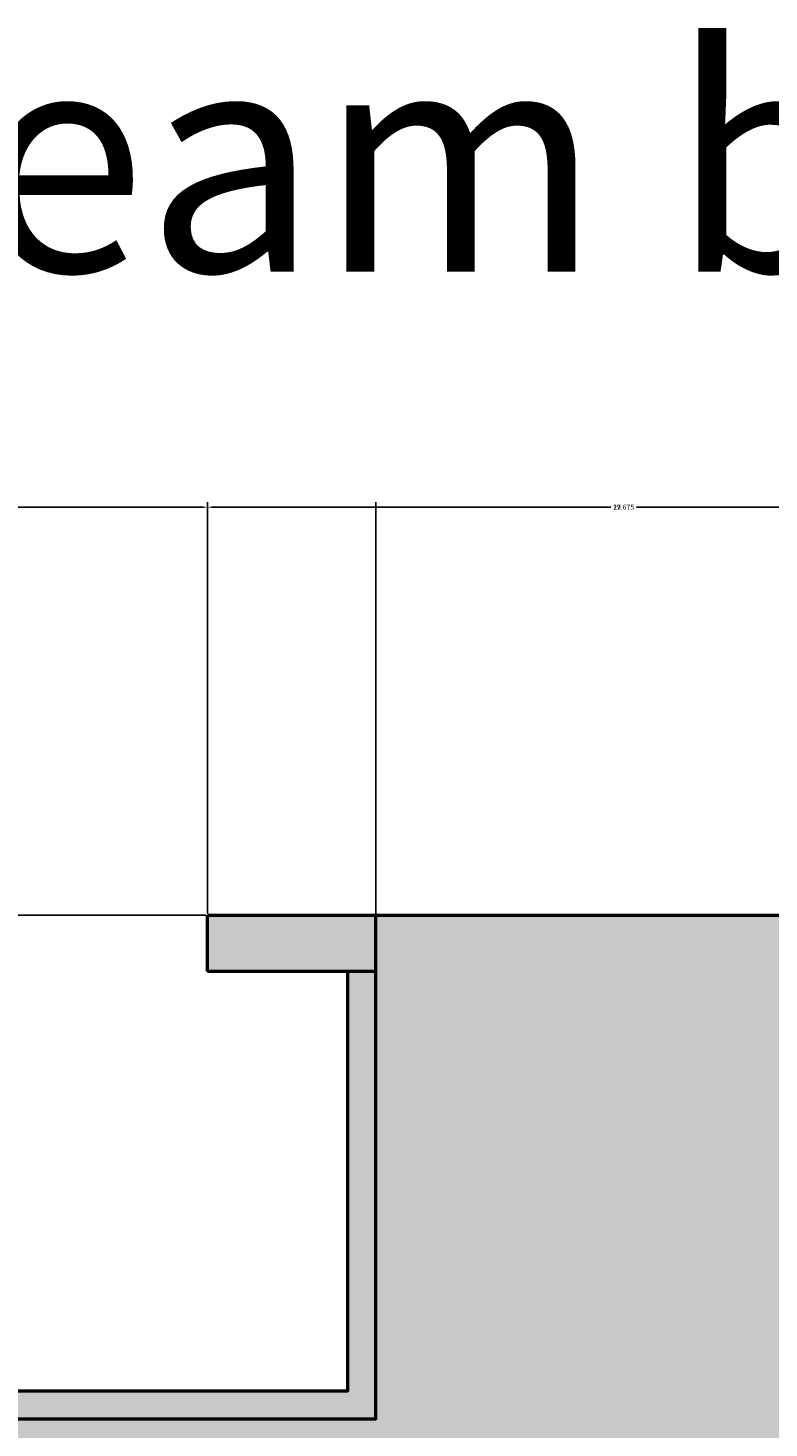
# Model space of a CAD drawing. Units: inches. Extents: x -12 to 334, y -10 to 186.
# Tile 66 of 77: x 184 to 210, y 137 to 186. Entities that reach past the tile are written whole.
import ezdxf

# ---------------------------------------------------------------- set-up
doc = ezdxf.new("R2010")
doc.units = ezdxf.units.IN
doc.header["$MEASUREMENT"] = 0
for name, color, linetype, lineweight in [('M-ANNO-TEXT', 3, 'Continuous', 25), ('M-DIMS', 2, 'Continuous', 18), ('M-EQPM', 7, 'Continuous', 50), ('M-EQPM-PATT', 8, 'Continuous', 18)]:
    doc.layers.add(name, color=color, linetype=linetype, lineweight=lineweight)
doc.styles.get("Standard").update_dxf_attribs({"font": 'arial.ttf'})
doc.dimstyles.get("Standard").update_dxf_attribs({"dimtxt": 0.18, "dimasz": 0.18, "dimexe": 0.18, "dimexo": 0.0625, "dimgap": 0.09, "dimtad": 0, "dimtih": 1, "dimtoh": 1, "dimdec": 4, "dimzin": 0, "dimdsep": 46, "dimtxsty": 'Standard', "dimcen": 0.09, "dimadec": 0, "dimazin": 0, "dimtfac": 1, "dimtdec": 4, "dimtofl": 0, "dimtmove": 0, "dimatfit": 3, "dimfxl": 1, "dimtolj": 1, "dimtzin": 0, "dimarcsym": 0})

# ---------------------------------------------------------------- blocks, each defined once
blk = doc.blocks.new('*D18')
at = {"layer": 'Defpoints', "color": 0, "transparency": 16777216}
for p in [(190.342, 169.385), (190.342, 154.835), (126.379, 137.887)]:
    blk.add_point(p, dxfattribs=at)
at = {"layer": 'M-DIMS', "color": 0, "lineweight": -2, "transparency": 16777216}
for p, q in [((126.379, 137.95), (126.379, 169.565)), ((126.559, 169.385), (157.967, 169.385)), ((190.162, 169.385), (158.755, 169.385)), ((190.342, 154.897), (190.342, 169.565))]:
    blk.add_line(p, q, dxfattribs=at)
at = {"layer": 'M-DIMS', "color": 0, "transparency": 16777216}
for points in [[(126.559, 169.415), (126.559, 169.355), (126.379, 169.385)], [(190.162, 169.415), (190.162, 169.355), (190.342, 169.385)]]:
    blk.add_solid(points, dxfattribs=at)
at = {"layer": 'M-DIMS', "color": 0, "transparency": 16777216, "insert": (158.361, 169.385), "char_height": 0.18, "attachment_point": 5}
blk.add_mtext('\\A1;63.96', dxfattribs=at)
blk = doc.blocks.new('*D19')
at = {"layer": 'Defpoints', "color": 0, "transparency": 16777216}
for p in [(220.017, 169.385), (190.342, 154.835), (220.017, 154.835)]:
    blk.add_point(p, dxfattribs=at)
at = {"layer": 'M-DIMS', "color": 0, "lineweight": -2, "transparency": 16777216}
for p, q in [((190.342, 154.897), (190.342, 169.565)), ((190.522, 169.385), (204.714, 169.385)), ((219.837, 169.385), (205.645, 169.385)), ((220.017, 154.897), (220.017, 169.565))]:
    blk.add_line(p, q, dxfattribs=at)
at = {"layer": 'M-DIMS', "color": 0, "transparency": 16777216}
for points in [[(190.522, 169.415), (190.522, 169.355), (190.342, 169.385)], [(219.837, 169.415), (219.837, 169.355), (220.017, 169.385)]]:
    blk.add_solid(points, dxfattribs=at)
at = {"layer": 'M-DIMS', "color": 0, "transparency": 16777216, "insert": (205.179, 169.385), "char_height": 0.18, "attachment_point": 5}
blk.add_mtext('\\A1;29.675', dxfattribs=at)
blk = doc.blocks.new('*D20')
at = {"layer": 'Defpoints', "color": 0, "transparency": 16777216}
for p in [(214.017, 169.385), (196.342, 154.835), (214.017, 154.835)]:
    blk.add_point(p, dxfattribs=at)
at = {"layer": 'M-DIMS', "color": 0, "lineweight": -2, "transparency": 16777216}
for p, q in [((196.342, 154.897), (196.342, 169.565)), ((196.522, 169.385), (204.724, 169.385)), ((213.837, 169.385), (205.635, 169.385)), ((214.017, 154.897), (214.017, 169.565))]:
    blk.add_line(p, q, dxfattribs=at)
at = {"layer": 'M-DIMS', "color": 0, "transparency": 16777216}
for points in [[(196.522, 169.415), (196.522, 169.355), (196.342, 169.385)], [(213.837, 169.415), (213.837, 169.355), (214.017, 169.385)]]:
    blk.add_solid(points, dxfattribs=at)
at = {"layer": 'M-DIMS', "color": 0, "transparency": 16777216, "insert": (205.179, 169.385), "char_height": 0.18, "attachment_point": 5}
blk.add_mtext('\\A1;17.675', dxfattribs=at)
blk = doc.blocks.new('*D22')
at = {"layer": 'Defpoints', "color": 0, "transparency": 16777216}
for p in [(190.342, 154.835), (-11.174, 137.887), (195.342, 137.887)]:
    blk.add_point(p, dxfattribs=at)
at = {"layer": 'M-DIMS', "color": 0, "lineweight": -2, "transparency": 16777216}
for p, q in [((190.28, 154.835), (-11.354, 154.835)), ((-11.174, 154.655), (-11.174, 146.543)), ((-11.174, 138.067), (-11.174, 146.179)), ((195.28, 137.887), (-11.354, 137.887))]:
    blk.add_line(p, q, dxfattribs=at)
at = {"layer": 'M-DIMS', "color": 0, "transparency": 16777216}
for points in [[(-11.204, 154.655), (-11.144, 154.655), (-11.174, 154.835)], [(-11.204, 138.067), (-11.144, 138.067), (-11.174, 137.887)]]:
    blk.add_solid(points, dxfattribs=at)
at = {"layer": 'M-DIMS', "color": 0, "transparency": 16777216, "insert": (-11.174, 146.361), "char_height": 0.18, "attachment_point": 5}
blk.add_mtext('\\A1;16.947', dxfattribs=at)

msp = doc.modelspace()

# ---------------------------------------------------------------- hatches: boundary and pattern name
at = {"layer": 'M-EQPM-PATT', "transparency": 33554556}
h = msp.add_hatch(color=256, dxfattribs=at)
h.set_gradient(color1=(248, 206, 179), color2=(248, 206, 179), tint=1)
h.paths.add_polyline_path([(179.7818, 136.8871), (126.9567, 136.8871), (106.1771, 100.8958), (171.5458, 100.8958)])
h.paths.add_polyline_path([(268.3808, 136.9435), (214.0166, 136.9435), (214.0166, 154.8345), (196.3421, 154.8345), (196.3421, 136.8871), (179.7818, 136.8871), (171.5458, 100.8958), (231.7758, 100.8958, -0.4142136), (251.9801, 80.6915), (279.7263, 80.6915, 0.1631825)])
at = {"layer": 'M-EQPM-PATT'}
h = msp.add_hatch(color=256, dxfattribs=at)
h.set_gradient(color1=(99, 100, 102), color2=(99, 100, 102), tint=1)
h.paths.add_polyline_path([(190.3421, 154.8345), (190.3421, 152.8345), (196.3421, 152.8345), (196.3421, 154.8345)])
h.paths.add_polyline_path([(220.0166, 152.8345), (220.0166, 154.8345), (214.0166, 154.8345), (214.0166, 152.8345)])
h = msp.add_hatch(color=256, dxfattribs=at)
h.set_gradient(color1=(99, 100, 102), color2=(99, 100, 102), tint=1)
h.paths.add_polyline_path([(126.9567, 136.8871), (179.7818, 136.8871), (180.0106, 137.8871), (126.3793, 137.8871), (106.1771, 102.8958), (86.8879, 102.8958), (86.8879, 109.0583), (84.7229, 109.0583), (84.7229, 100.8958), (106.1771, 100.8958)])
h.paths.add_polyline_path([(196.3421, 152.8345), (195.3421, 152.8345), (195.3421, 137.8871), (180.0106, 137.8871), (179.7818, 136.8871), (196.3421, 136.8871)])
h.paths.add_polyline_path([(215.0166, 152.8345), (214.0166, 152.8345), (214.0166, 136.9435), (268.3808, 136.9435, -0.2673785), (268.3808, 46.8541), (249.3759, 46.8541), (249.8485, 45.8541), (269.3808, 45.8541, 0.2615891), (269.3808, 137.9435), (215.0166, 137.9435)])

# ---------------------------------------------------------------- linework, layer by layer
at = {"layer": 'M-EQPM'}
for p, q in [((190.3421, 152.8345), (190.3421, 154.8345)), ((190.3421, 154.8345), (220.0166, 154.8345)), ((196.3421, 152.8345), (190.3421, 152.8345))]:
    msp.add_line(p, q, dxfattribs=at)
for points in [[(106.1771, 100.8958), (126.9567, 136.8871), (196.3421, 136.8871), (196.3421, 154.8345)], [(106.1771, 102.8958), (126.3793, 137.8871), (195.3421, 137.8871), (195.3421, 152.8345)]]:
    msp.add_lwpolyline(points, dxfattribs=at)

# ---------------------------------------------------------------- texts
at = {"layer": 'M-ANNO-TEXT', "insert": (70.1252, 185.7805), "char_height": 8, "attachment_point": 1}
msp.add_mtext_dynamic_manual_height_columns('Heat exchanger in a steam boiler', width=205.597506, gutter_width=1, heights=[0], dxfattribs=at)

# ---------------------------------------------------------------- dimensions: what is measured, and where the dimension line sits
at = {"layer": 'M-DIMS'}
for base, p1, p2, override, picture, middle in [((190.3421, 169.3845), (126.3793, 137.8871), (190.3421, 154.8345), {"dimdec": 2, "dimlfac": 1, "dimrnd": 0, "dimzin": 0, "dimdsep": 46, "dimlunit": 2}, '*D18', (158.3607, 169.3845)), ((220.01662, 169.38453), (190.34209, 154.83453), (220.01662, 154.83453), {"dimdec": 3, "dimlfac": 1, "dimrnd": 0, "dimzin": 0, "dimdsep": 46, "dimlunit": 2}, '*D19', (205.17936, 169.38453)), ((214.01662, 169.38453), (196.34209, 154.83453), (214.01662, 154.83453), {"dimdec": 3, "dimlfac": 1, "dimrnd": 0, "dimzin": 0, "dimdsep": 46, "dimlunit": 2}, '*D20', (205.17936, 169.38453))]:
    dim = msp.add_linear_dim(base=base, p1=p1, p2=p2, dimstyle='Standard', override=override, dxfattribs=at)
    dim.commit()
    dim.dimension.update_dxf_attribs({"geometry": picture, "text_midpoint": middle})
dim = msp.add_linear_dim(base=(-11.1736, 137.8871), p1=(190.3421, 154.8345), p2=(195.3421, 137.8871), angle=90, dimstyle='Standard', override={"dimdec": 3, "dimlfac": 1, "dimrnd": 0, "dimzin": 0, "dimdsep": 46, "dimlunit": 2}, dxfattribs=at)
dim.commit()
dim.dimension.update_dxf_attribs({"geometry": '*D22', "text_midpoint": (-11.1735, 146.3608)})

doc.saveas('drawing.dxf')
